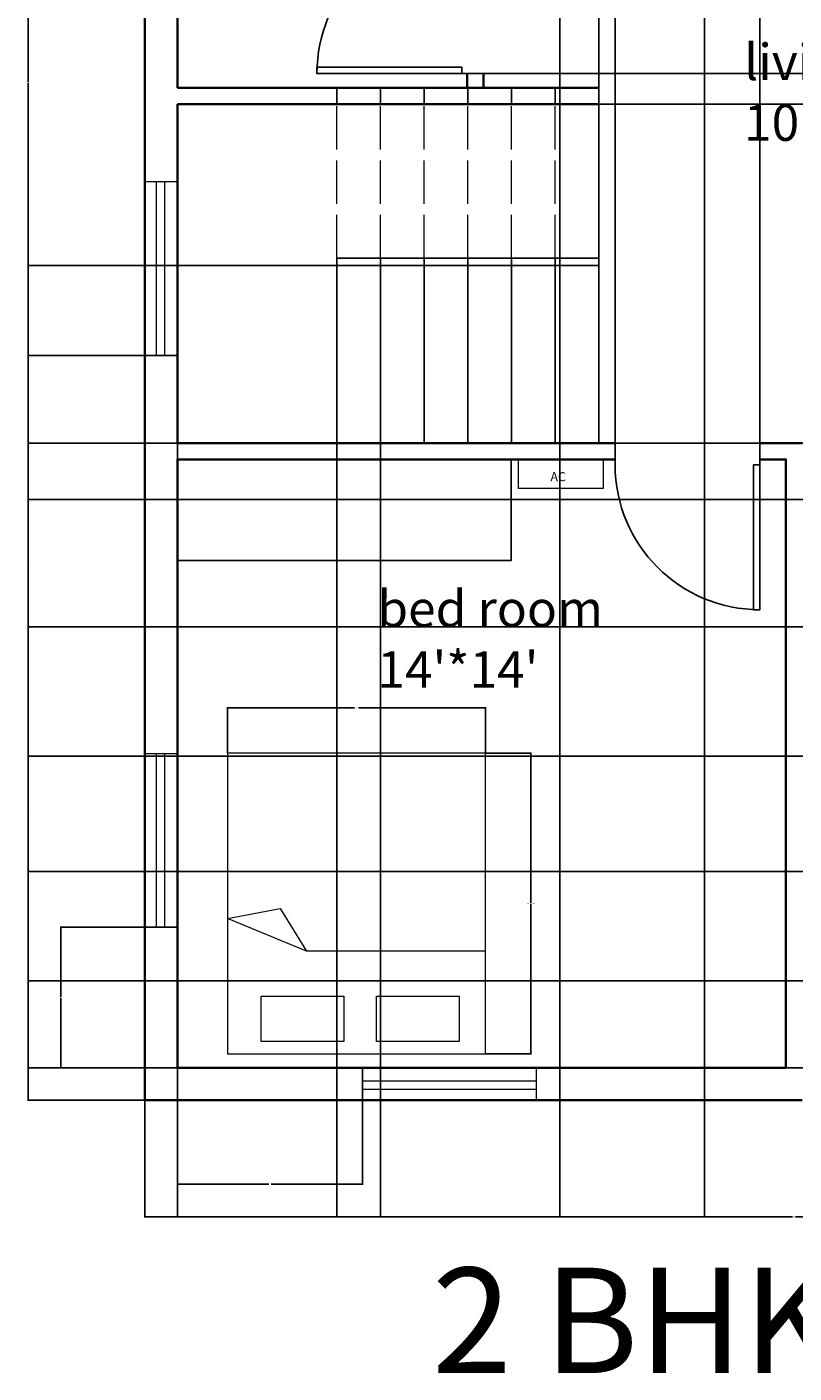
# Model space of a CAD drawing. Units: inches. Extents: x 2187 to 2611, y 763 to 1433.
# Tile 1 of 3: x 2187 to 2399, y 763 to 1135. Entities that reach past the tile are written whole.
import ezdxf

# ---------------------------------------------------------------- set-up
doc = ezdxf.new("R2010")
doc.units = ezdxf.units.IN
doc.linetypes.add('ACAD_ISO02W100', pattern=[15, 12, -3])
for name, color, linetype, lineweight in [('A-ANNO-DIMS', 2, 'Continuous', 18), ('A-ANNO-TEXT', 7, 'Continuous', 18), ('A-ANNO-TITL', 7, 'Continuous', 35), ('A-AREA-IDEN', 7, 'Continuous', 18), ('A-FLOR-CASE', 82, 'Continuous', 25), ('A-FLOR-STRS', 7, 'Continuous', 25), ('A-FLOR-STRS-OVHD', 7, 'ACAD_ISO02W100', 18), ('A-WALL', 7, 'Continuous', 35), ('DOOR', 130, 'Continuous', 25), ('FURNITURE', 82, 'Continuous', 18), ('M-HVAC-EQPM', 82, 'Continuous', 18), ('WINDOW', 50, 'Continuous', 20)]:
    doc.layers.add(name, color=color, linetype=linetype, lineweight=lineweight)
doc.styles.get("Standard").update_dxf_attribs({"font": 'arial.ttf'})
doc.dimstyles.get("Standard").update_dxf_attribs({"dimtxt": 0.18, "dimasz": 0.18, "dimexe": 0.18, "dimexo": 0.0625, "dimgap": 0.09, "dimtad": 0, "dimtih": 1, "dimtoh": 1, "dimdec": 4, "dimzin": 0, "dimdsep": 46, "dimtxsty": 'Standard', "dimcen": 0.09, "dimadec": 0, "dimazin": 0, "dimtfac": 1, "dimtdec": 4, "dimtofl": 0, "dimtmove": 0, "dimatfit": 3, "dimfxl": 1, "dimtolj": 1, "dimtzin": 0, "dimarcsym": 0})

# ---------------------------------------------------------------- blocks, each defined once
blk = doc.blocks.new('*U2')
for p, q in [((0, 0), (0, -6)), ((40, 0), (40, -6))]:
    blk.add_line(p, q)
blk.add_lwpolyline([(0, 0), (0, 40), (1.75, 40), (1.75, 0)], close=True)
blk.add_arc((0, 0), 40, 0, 90)
blk = doc.blocks.new('BED-DOUBLE')
for p, q in [((54.72, 71.29), (54.72, 21.8)), ((42.94, 14.53), (54.72, 21.8)), ((54.72, 21.8), (45.71, 0)), ((45.71, 0), (42.94, 14.53))]:
    blk.add_line(p, q)
for points in [[(83.12, 71.29), (0, 71.29), (0, 0), (83.12, 0)], [(67.19, 64.02), (79.65, 64.02), (79.65, 41.18), (67.19, 41.18)], [(67.19, 32.18), (79.65, 32.18), (79.65, 9.34), (67.19, 9.34)]]:
    blk.add_lwpolyline(points, close=True)
blk = doc.blocks.new('WIN-48IN')
for p, q in [((0, 0), (0, 9)), ((48, 0), (48, 9)), ((0, 5.37), (48, 5.37)), ((0, 3.09), (48, 3.09))]:
    blk.add_line(p, q)
blk = doc.blocks.new('*D10')
at = {"layer": 'A-ANNO-DIMS', "color": 0, "lineweight": -2, "transparency": 16777216}
for p, q in [((2313.9, 934.72), (2326.49, 934.72)), ((2326.31, 934.54), (2326.31, 893.34)), ((2326.31, 851.78), (2326.31, 892.98)), ((2313.9, 851.6), (2326.49, 851.6))]:
    blk.add_line(p, q, dxfattribs=at)
at = {"layer": 'A-ANNO-DIMS', "color": 0, "lineweight": 100, "transparency": 16777216}
for points in [[(2326.28, 934.54), (2326.34, 934.54), (2326.31, 934.72)], [(2326.28, 851.78), (2326.34, 851.78), (2326.31, 851.6)]]:
    blk.add_solid(points, dxfattribs=at)
at = {"layer": 'Defpoints', "color": 0, "lineweight": 100, "transparency": 16777216}
for p in [(2313.84, 934.72), (2313.84, 851.6), (2326.31, 851.6)]:
    blk.add_point(p, dxfattribs=at)
at = {"layer": 'A-ANNO-DIMS', "color": 0, "transparency": 16777216, "insert": (2326.31, 893.16), "char_height": 0.18, "attachment_point": 5}
blk.add_mtext('\\A1;DOUBLE BED 83 TYP.', dxfattribs=at)
blk = doc.blocks.new('*D11')
at = {"layer": 'A-ANNO-DIMS', "color": 0, "lineweight": -2, "transparency": 16777216}
for p, q in [((2242.55, 934.78), (2242.55, 947.37)), ((2242.73, 947.19), (2277.67, 947.19)), ((2313.66, 947.19), (2278.72, 947.19)), ((2313.84, 934.78), (2313.84, 947.37))]:
    blk.add_line(p, q, dxfattribs=at)
at = {"layer": 'A-ANNO-DIMS', "color": 0, "lineweight": 100, "transparency": 16777216}
for points in [[(2242.73, 947.22), (2242.73, 947.16), (2242.55, 947.19)], [(2313.66, 947.22), (2313.66, 947.16), (2313.84, 947.19)]]:
    blk.add_solid(points, dxfattribs=at)
at = {"layer": 'Defpoints', "color": 0, "lineweight": 100, "transparency": 16777216}
for p in [(2313.84, 947.19), (2242.55, 934.72), (2313.84, 934.72)]:
    blk.add_point(p, dxfattribs=at)
at = {"layer": 'A-ANNO-DIMS', "color": 0, "transparency": 16777216, "insert": (2278.2, 947.19), "char_height": 0.18, "attachment_point": 5}
blk.add_mtext('\\A1;71 TYP.', dxfattribs=at)
blk = doc.blocks.new('*D14')
at = {"layer": 'A-ANNO-DIMS', "color": 0, "lineweight": -2, "transparency": 16777216}
for p, q in [((2219.77, 838.73), (2219.77, 806.41)), ((2578.27, 838.73), (2578.27, 806.41)), ((2219.95, 806.59), (2398.62, 806.59)), ((2578.09, 806.59), (2399.41, 806.59))]:
    blk.add_line(p, q, dxfattribs=at)
at = {"layer": 'A-ANNO-DIMS', "color": 0, "lineweight": 100, "transparency": 16777216}
for points in [[(2219.95, 806.62), (2219.95, 806.56), (2219.77, 806.59)], [(2578.09, 806.62), (2578.09, 806.56), (2578.27, 806.59)]]:
    blk.add_solid(points, dxfattribs=at)
at = {"layer": 'Defpoints', "color": 0, "lineweight": 100, "transparency": 16777216}
for p in [(2219.77, 838.79), (2578.27, 838.79), (2578.27, 806.59)]:
    blk.add_point(p, dxfattribs=at)
at = {"layer": 'A-ANNO-DIMS', "color": 0, "transparency": 16777216, "insert": (2399.02, 806.59), "char_height": 0.18, "attachment_point": 5}
blk.add_mtext('\\A1;358.5', dxfattribs=at)
blk = doc.blocks.new('*D15')
at = {"layer": 'A-ANNO-DIMS', "color": 0, "lineweight": -2, "transparency": 16777216}
for p, q in [((2219.71, 1400.96), (2187.39, 1400.96)), ((2187.57, 1400.78), (2187.57, 1120.06)), ((2187.57, 838.97), (2187.57, 1119.7)), ((2219.71, 838.79), (2187.39, 838.79))]:
    blk.add_line(p, q, dxfattribs=at)
at = {"layer": 'A-ANNO-DIMS', "color": 0, "lineweight": 100, "transparency": 16777216}
for points in [[(2187.54, 1400.78), (2187.6, 1400.78), (2187.57, 1400.96)], [(2187.54, 838.97), (2187.6, 838.97), (2187.57, 838.79)]]:
    blk.add_solid(points, dxfattribs=at)
at = {"layer": 'Defpoints', "color": 0, "lineweight": 100, "transparency": 16777216}
for p in [(2187.57, 1400.96), (2219.77, 1400.96), (2219.77, 838.79)]:
    blk.add_point(p, dxfattribs=at)
at = {"layer": 'A-ANNO-DIMS', "color": 0, "transparency": 16777216, "insert": (2187.57, 1119.88), "char_height": 0.18, "attachment_point": 5}
blk.add_mtext('\\A1;562.2', dxfattribs=at)
blk = doc.blocks.new('*D20')
at = {"layer": 'A-ANNO-DIMS', "color": 0, "lineweight": -2, "transparency": 16777216}
for p, q in [((2228.71, 886.61), (2196.39, 886.61)), ((2196.57, 886.43), (2196.57, 867.38)), ((2196.57, 847.97), (2196.57, 867.02)), ((2228.71, 847.79), (2196.39, 847.79))]:
    blk.add_line(p, q, dxfattribs=at)
at = {"layer": 'A-ANNO-DIMS', "color": 0, "lineweight": 100, "transparency": 16777216}
for points in [[(2196.54, 886.43), (2196.6, 886.43), (2196.57, 886.61)], [(2196.54, 847.97), (2196.6, 847.97), (2196.57, 847.79)]]:
    blk.add_solid(points, dxfattribs=at)
at = {"layer": 'Defpoints', "color": 0, "lineweight": 100, "transparency": 16777216}
for p in [(2196.57, 886.61), (2228.77, 886.61), (2228.77, 847.79)]:
    blk.add_point(p, dxfattribs=at)
at = {"layer": 'A-ANNO-DIMS', "color": 0, "transparency": 16777216, "insert": (2196.57, 867.2), "char_height": 0.18, "attachment_point": 5}
blk.add_mtext('\\A1;38.81', dxfattribs=at)
blk = doc.blocks.new('*D21')
at = {"layer": 'A-ANNO-DIMS', "color": 0, "lineweight": -2, "transparency": 16777216}
for p, q in [((2228.77, 847.73), (2228.77, 815.41)), ((2279.87, 847.73), (2279.87, 815.41)), ((2228.95, 815.59), (2254.01, 815.59)), ((2279.69, 815.59), (2254.63, 815.59))]:
    blk.add_line(p, q, dxfattribs=at)
at = {"layer": 'A-ANNO-DIMS', "color": 0, "lineweight": 100, "transparency": 16777216}
for points in [[(2228.95, 815.62), (2228.95, 815.56), (2228.77, 815.59)], [(2279.69, 815.62), (2279.69, 815.56), (2279.87, 815.59)]]:
    blk.add_solid(points, dxfattribs=at)
at = {"layer": 'Defpoints', "color": 0, "lineweight": 100, "transparency": 16777216}
for p in [(2228.77, 847.79), (2279.87, 847.79), (2228.77, 815.59)]:
    blk.add_point(p, dxfattribs=at)
at = {"layer": 'A-ANNO-DIMS', "color": 0, "transparency": 16777216, "insert": (2254.32, 815.59), "char_height": 0.18, "attachment_point": 5}
blk.add_mtext('\\A1;51.1', dxfattribs=at)
blk = doc.blocks.new('*D28')
at = {"layer": 'A-ANNO-DIMS', "color": 0, "lineweight": -2, "transparency": 16777216}
for p, q in [((2349.61, 1016.11), (2349.61, 1433.34)), ((2349.79, 1433.16), (2369.39, 1433.16)), ((2389.43, 1433.16), (2369.83, 1433.16)), ((2389.61, 1016.11), (2389.61, 1433.34))]:
    blk.add_line(p, q, dxfattribs=at)
at = {"layer": 'A-ANNO-DIMS', "color": 0, "lineweight": 100, "transparency": 16777216}
for points in [[(2349.79, 1433.19), (2349.79, 1433.13), (2349.61, 1433.16)], [(2389.43, 1433.19), (2389.43, 1433.13), (2389.61, 1433.16)]]:
    blk.add_solid(points, dxfattribs=at)
at = {"layer": 'Defpoints', "color": 0, "lineweight": 100, "transparency": 16777216}
for p in [(2389.61, 1433.16), (2349.61, 1016.04), (2389.61, 1016.04)]:
    blk.add_point(p, dxfattribs=at)
at = {"layer": 'A-ANNO-DIMS', "color": 0, "transparency": 16777216, "insert": (2369.61, 1433.16), "char_height": 0.18, "attachment_point": 5}
blk.add_mtext('\\A1;40', dxfattribs=at)
blk = doc.blocks.new('*D29')
at = {"layer": 'A-ANNO-DIMS', "color": 0, "lineweight": -2, "transparency": 16777216}
for p, q in [((2447.71, 1004.76), (2187.39, 1004.76)), ((2187.57, 1004.58), (2187.57, 987.33)), ((2187.57, 969.72), (2187.57, 986.97)), ((2447.71, 969.54), (2187.39, 969.54))]:
    blk.add_line(p, q, dxfattribs=at)
at = {"layer": 'A-ANNO-DIMS', "color": 0, "lineweight": 100, "transparency": 16777216}
for points in [[(2187.54, 1004.58), (2187.6, 1004.58), (2187.57, 1004.76)], [(2187.54, 969.72), (2187.6, 969.72), (2187.57, 969.54)]]:
    blk.add_solid(points, dxfattribs=at)
at = {"layer": 'Defpoints', "color": 0, "lineweight": 100, "transparency": 16777216}
for p in [(2187.57, 1004.76), (2447.77, 1004.76), (2447.77, 969.54)]:
    blk.add_point(p, dxfattribs=at)
at = {"layer": 'A-ANNO-DIMS', "color": 0, "transparency": 16777216, "insert": (2187.57, 987.15), "char_height": 0.18, "attachment_point": 5}
blk.add_mtext('\\A1;35.22', dxfattribs=at)
blk = doc.blocks.new('*D30')
at = {"layer": 'A-ANNO-DIMS', "color": 0, "lineweight": -2, "transparency": 16777216}
for p, q in [((2334.33, 1219.4), (2334.33, 806.41)), ((2374.33, 1219.4), (2374.33, 806.41)), ((2334.51, 806.59), (2354.11, 806.59)), ((2374.15, 806.59), (2354.56, 806.59))]:
    blk.add_line(p, q, dxfattribs=at)
at = {"layer": 'A-ANNO-DIMS', "color": 0, "lineweight": 100, "transparency": 16777216}
for points in [[(2334.51, 806.62), (2334.51, 806.56), (2334.33, 806.59)], [(2374.15, 806.62), (2374.15, 806.56), (2374.33, 806.59)]]:
    blk.add_solid(points, dxfattribs=at)
at = {"layer": 'Defpoints', "color": 0, "lineweight": 100, "transparency": 16777216}
for p in [(2334.33, 1219.46), (2374.33, 1219.46), (2374.33, 806.59)]:
    blk.add_point(p, dxfattribs=at)
at = {"layer": 'A-ANNO-DIMS', "color": 0, "transparency": 16777216, "insert": (2354.33, 806.59), "char_height": 0.18, "attachment_point": 5}
blk.add_mtext('\\A1;40', dxfattribs=at)
blk = doc.blocks.new('*D31')
at = {"layer": 'A-ANNO-DIMS', "color": 0, "lineweight": -2, "transparency": 16777216}
for p, q in [((2313.33, 1162.4), (2610.65, 1162.4)), ((2610.47, 1162.22), (2610.47, 1142.58)), ((2610.47, 1122.58), (2610.47, 1142.22)), ((2313.33, 1122.4), (2610.65, 1122.4))]:
    blk.add_line(p, q, dxfattribs=at)
at = {"layer": 'A-ANNO-DIMS', "color": 0, "lineweight": 100, "transparency": 16777216}
for points in [[(2610.44, 1162.22), (2610.5, 1162.22), (2610.47, 1162.4)], [(2610.44, 1122.58), (2610.5, 1122.58), (2610.47, 1122.4)]]:
    blk.add_solid(points, dxfattribs=at)
at = {"layer": 'Defpoints', "color": 0, "lineweight": 100, "transparency": 16777216}
for p in [(2313.27, 1162.4), (2610.47, 1162.4), (2313.27, 1122.4)]:
    blk.add_point(p, dxfattribs=at)
at = {"layer": 'A-ANNO-DIMS', "color": 0, "transparency": 16777216, "insert": (2610.47, 1142.4), "char_height": 0.18, "attachment_point": 5}
blk.add_mtext('\\A1;40', dxfattribs=at)
blk = doc.blocks.new('*D34')
at = {"layer": 'A-ANNO-DIMS', "color": 0, "lineweight": -2, "transparency": 16777216}
for p, q in [((2449.71, 871.79), (2187.39, 871.79)), ((2187.57, 871.61), (2187.57, 859.97)), ((2187.57, 847.97), (2187.57, 859.61)), ((2449.71, 847.79), (2187.39, 847.79))]:
    blk.add_line(p, q, dxfattribs=at)
at = {"layer": 'A-ANNO-DIMS', "color": 0, "lineweight": 100, "transparency": 16777216}
for points in [[(2187.54, 871.61), (2187.6, 871.61), (2187.57, 871.79)], [(2187.54, 847.97), (2187.6, 847.97), (2187.57, 847.79)]]:
    blk.add_solid(points, dxfattribs=at)
at = {"layer": 'Defpoints', "color": 0, "lineweight": 100, "transparency": 16777216}
for p in [(2187.57, 871.79), (2449.78, 871.79), (2449.78, 847.79)]:
    blk.add_point(p, dxfattribs=at)
at = {"layer": 'A-ANNO-DIMS', "color": 0, "transparency": 16777216, "insert": (2187.57, 859.79), "char_height": 0.18, "attachment_point": 5}
blk.add_mtext('\\A1;24', dxfattribs=at)
blk = doc.blocks.new('*D43')
at = {"layer": 'A-ANNO-DIMS', "color": 0, "lineweight": -2, "transparency": 16777216}
for p, q in [((2546.13, 933.87), (2187.39, 933.87)), ((2187.57, 933.69), (2187.57, 918.13)), ((2187.57, 902.21), (2187.57, 917.77)), ((2546.13, 902.03), (2187.39, 902.03))]:
    blk.add_line(p, q, dxfattribs=at)
at = {"layer": 'A-ANNO-DIMS', "color": 0, "lineweight": 100, "transparency": 16777216}
for points in [[(2187.54, 933.69), (2187.6, 933.69), (2187.57, 933.87)], [(2187.54, 902.21), (2187.6, 902.21), (2187.57, 902.03)]]:
    blk.add_solid(points, dxfattribs=at)
at = {"layer": 'Defpoints', "color": 0, "lineweight": 100, "transparency": 16777216}
for p in [(2187.57, 933.87), (2546.19, 933.87), (2546.19, 902.03)]:
    blk.add_point(p, dxfattribs=at)
at = {"layer": 'A-ANNO-DIMS', "color": 0, "transparency": 16777216, "insert": (2187.57, 917.95), "char_height": 0.18, "attachment_point": 5}
blk.add_mtext('\\A1;31.837', dxfattribs=at)
blk = doc.blocks.new('*D44')
at = {"layer": 'A-ANNO-DIMS', "color": 0, "lineweight": -2, "transparency": 16777216}
for p, q in [((2228.77, 1118.52), (2228.77, 1433.34)), ((2228.95, 1433.16), (2286.53, 1433.16)), ((2344.89, 1433.16), (2287.3, 1433.16)), ((2345.07, 1118.52), (2345.07, 1433.34))]:
    blk.add_line(p, q, dxfattribs=at)
at = {"layer": 'A-ANNO-DIMS', "color": 0, "lineweight": 100, "transparency": 16777216}
for points in [[(2228.95, 1433.19), (2228.95, 1433.13), (2228.77, 1433.16)], [(2344.89, 1433.19), (2344.89, 1433.13), (2345.07, 1433.16)]]:
    blk.add_solid(points, dxfattribs=at)
at = {"layer": 'Defpoints', "color": 0, "lineweight": 100, "transparency": 16777216}
for p in [(2345.07, 1433.16), (2228.77, 1118.46), (2345.07, 1118.46)]:
    blk.add_point(p, dxfattribs=at)
at = {"layer": 'A-ANNO-DIMS', "color": 0, "transparency": 16777216, "insert": (2286.92, 1433.16), "char_height": 0.18, "attachment_point": 5}
blk.add_mtext('\\A1;116.3', dxfattribs=at)
blk = doc.blocks.new('*D45')
at = {"layer": 'A-ANNO-DIMS', "color": 0, "lineweight": -2, "transparency": 16777216}
for p, q in [((2345.13, 1113.96), (2610.65, 1113.96)), ((2610.47, 1113.78), (2610.47, 1067.31)), ((2610.47, 1020.47), (2610.47, 1066.94)), ((2345.13, 1020.29), (2610.65, 1020.29))]:
    blk.add_line(p, q, dxfattribs=at)
at = {"layer": 'A-ANNO-DIMS', "color": 0, "lineweight": 100, "transparency": 16777216}
for points in [[(2610.44, 1113.78), (2610.5, 1113.78), (2610.47, 1113.96)], [(2610.44, 1020.47), (2610.5, 1020.47), (2610.47, 1020.29)]]:
    blk.add_solid(points, dxfattribs=at)
at = {"layer": 'Defpoints', "color": 0, "lineweight": 100, "transparency": 16777216}
for p in [(2345.07, 1113.96), (2610.47, 1113.96), (2345.07, 1020.29)]:
    blk.add_point(p, dxfattribs=at)
at = {"layer": 'A-ANNO-DIMS', "color": 0, "transparency": 16777216, "insert": (2610.47, 1067.13), "char_height": 0.18, "attachment_point": 5}
blk.add_mtext('\\A1;93.67', dxfattribs=at)
blk = doc.blocks.new('*D46')
at = {"layer": 'A-ANNO-DIMS', "color": 0, "lineweight": -2, "transparency": 16777216}
for p, q in [((2228.77, 1020.23), (2228.77, 806.41)), ((2272.77, 1020.23), (2272.77, 806.41)), ((2228.95, 806.59), (2250.55, 806.59)), ((2272.59, 806.59), (2250.99, 806.59))]:
    blk.add_line(p, q, dxfattribs=at)
at = {"layer": 'A-ANNO-DIMS', "color": 0, "lineweight": 100, "transparency": 16777216}
for points in [[(2228.95, 806.62), (2228.95, 806.56), (2228.77, 806.59)], [(2272.59, 806.62), (2272.59, 806.56), (2272.77, 806.59)]]:
    blk.add_solid(points, dxfattribs=at)
at = {"layer": 'Defpoints', "color": 0, "lineweight": 100, "transparency": 16777216}
for p in [(2228.77, 1020.29), (2272.77, 1020.29), (2272.77, 806.59)]:
    blk.add_point(p, dxfattribs=at)
at = {"layer": 'A-ANNO-DIMS', "color": 0, "transparency": 16777216, "insert": (2250.77, 806.59), "char_height": 0.18, "attachment_point": 5}
blk.add_mtext('\\A1;44', dxfattribs=at)
blk = doc.blocks.new('*D47')
at = {"layer": 'A-ANNO-DIMS', "color": 0, "lineweight": -2, "transparency": 16777216}
for p, q in [((2272.77, 1020.23), (2272.77, 806.41)), ((2284.82, 1020.23), (2284.82, 806.41)), ((2272.95, 806.59), (2278.41, 806.59)), ((2284.64, 806.59), (2279.18, 806.59))]:
    blk.add_line(p, q, dxfattribs=at)
at = {"layer": 'A-ANNO-DIMS', "color": 0, "lineweight": 100, "transparency": 16777216}
for points in [[(2272.95, 806.62), (2272.95, 806.56), (2272.77, 806.59)], [(2284.64, 806.62), (2284.64, 806.56), (2284.82, 806.59)]]:
    blk.add_solid(points, dxfattribs=at)
at = {"layer": 'Defpoints', "color": 0, "lineweight": 100, "transparency": 16777216}
for p in [(2272.77, 1020.29), (2284.82, 1020.29), (2284.82, 806.59)]:
    blk.add_point(p, dxfattribs=at)
at = {"layer": 'A-ANNO-DIMS', "color": 0, "transparency": 16777216, "insert": (2278.79, 806.59), "char_height": 0.18, "attachment_point": 5}
blk.add_mtext('\\A1;12.05', dxfattribs=at)
blk = doc.blocks.new('*D48')
at = {"layer": 'A-ANNO-DIMS', "color": 0, "lineweight": -2, "transparency": 16777216}
for p, q in [((2272.71, 1069.38), (2187.39, 1069.38)), ((2187.57, 1069.2), (2187.57, 1045.02)), ((2187.57, 1020.47), (2187.57, 1044.65)), ((2272.71, 1020.29), (2187.39, 1020.29))]:
    blk.add_line(p, q, dxfattribs=at)
at = {"layer": 'A-ANNO-DIMS', "color": 0, "lineweight": 100, "transparency": 16777216}
for points in [[(2187.54, 1069.2), (2187.6, 1069.2), (2187.57, 1069.38)], [(2187.54, 1020.47), (2187.6, 1020.47), (2187.57, 1020.29)]]:
    blk.add_solid(points, dxfattribs=at)
at = {"layer": 'Defpoints', "color": 0, "lineweight": 100, "transparency": 16777216}
for p in [(2187.57, 1069.38), (2272.77, 1069.38), (2272.77, 1020.29)]:
    blk.add_point(p, dxfattribs=at)
at = {"layer": 'A-ANNO-DIMS', "color": 0, "transparency": 16777216, "insert": (2187.57, 1044.84), "char_height": 0.18, "attachment_point": 5}
blk.add_mtext('\\A1;49.08', dxfattribs=at)
blk = doc.blocks.new('*D49')
at = {"layer": 'A-ANNO-DIMS', "color": 0, "lineweight": -2, "transparency": 16777216}
for p, q in [((2228.71, 1044.55), (2187.39, 1044.55)), ((2187.57, 1044.37), (2187.57, 1032.6)), ((2187.57, 1020.47), (2187.57, 1032.24)), ((2228.71, 1020.29), (2187.39, 1020.29))]:
    blk.add_line(p, q, dxfattribs=at)
at = {"layer": 'A-ANNO-DIMS', "color": 0, "lineweight": 100, "transparency": 16777216}
for points in [[(2187.54, 1044.37), (2187.6, 1044.37), (2187.57, 1044.55)], [(2187.54, 1020.47), (2187.6, 1020.47), (2187.57, 1020.29)]]:
    blk.add_solid(points, dxfattribs=at)
at = {"layer": 'Defpoints', "color": 0, "lineweight": 100, "transparency": 16777216}
for p in [(2187.57, 1044.55), (2228.77, 1044.55), (2228.77, 1020.29)]:
    blk.add_point(p, dxfattribs=at)
at = {"layer": 'A-ANNO-DIMS', "color": 0, "transparency": 16777216, "insert": (2187.57, 1032.42), "char_height": 0.18, "attachment_point": 5}
blk.add_mtext('\\A1;24.25', dxfattribs=at)

msp = doc.modelspace()

# ---------------------------------------------------------------- linework, layer by layer
at = {"layer": 'A-FLOR-CASE'}
msp.add_lwpolyline([(2228.7681, 1015.7937), (2320.9466, 1015.7937), (2320.9466, 987.9063), (2228.7681, 987.9063)], close=True, dxfattribs=at)
at = {"layer": 'A-FLOR-STRS'}
for p, q in [((2272.7686, 1118.4602), (2272.7686, 1113.9602)), ((2284.8182, 1118.4602), (2284.8182, 1113.9602)), ((2296.8678, 1118.4602), (2296.8678, 1113.9602)), ((2308.9175, 1118.4602), (2308.9175, 1113.9602)), ((2320.9671, 1118.4602), (2320.9671, 1113.9602)), ((2333.0167, 1118.4602), (2333.0167, 1113.9602)), ((2345.0663, 1113.9602), (2345.0663, 1118.4602)), ((2345.0663, 1069.377), (2345.0663, 1118.4602)), ((2345.0663, 1118.4602), (2345.0663, 1020.2937)), ((2228.7681, 1113.9602), (2228.7681, 1020.2937)), ((2272.7686, 1071.377), (2345.0663, 1071.377)), ((2272.7686, 1071.377), (2272.7686, 1020.2937)), ((2284.8182, 1071.377), (2284.8182, 1020.2937)), ((2296.8678, 1071.377), (2296.8678, 1020.2937)), ((2308.9175, 1071.377), (2308.9175, 1020.2937)), ((2320.9671, 1071.377), (2320.9671, 1020.2937)), ((2333.0167, 1071.377), (2333.0167, 1020.2937)), ((2272.7686, 1069.377), (2345.0663, 1069.377))]:
    msp.add_line(p, q, dxfattribs=at)
at = {"layer": 'A-FLOR-STRS-OVHD'}
for p, q in [((2272.7686, 1071.377), (2272.7686, 1113.9602)), ((2284.8182, 1071.377), (2284.8182, 1113.9602)), ((2296.8678, 1071.377), (2296.8678, 1113.9602)), ((2308.9175, 1071.377), (2308.9175, 1113.9602)), ((2320.9671, 1071.377), (2320.9671, 1113.9602)), ((2333.0167, 1071.377), (2333.0167, 1113.9602))]:
    msp.add_line(p, q, dxfattribs=at)
at = {"layer": 'A-WALL'}
for p, q in [((2219.7681, 1118.4602), (2219.7681, 1223.9602)), ((2228.7681, 1118.4602), (2228.7681, 1219.4602)), ((2308.7681, 1122.3972), (2308.7681, 1118.4602)), ((2313.2681, 1122.3972), (2313.2681, 1118.4602)), ((2219.7681, 1020.2937), (2219.7681, 1118.4602)), ((2228.7681, 1118.4602), (2345.0663, 1118.4602)), ((2228.7681, 1020.2937), (2228.7681, 1113.9602)), ((2228.7681, 1113.9602), (2345.0663, 1113.9602)), ((2219.7681, 1020.2937), (2219.7681, 838.7937)), ((2228.7681, 1020.2937), (2349.6096, 1020.2937)), ((2389.6096, 1020.2937), (2401.2681, 1020.2937)), ((2228.7681, 1015.7937), (2349.6096, 1015.7937)), ((2228.7681, 1015.7937), (2228.7681, 847.7937)), ((2389.6096, 1015.7937), (2396.7681, 1015.7937)), ((2396.7681, 847.7937), (2396.7681, 1015.7937)), ((2228.7681, 847.7937), (2396.7681, 847.7937)), ((2219.7681, 838.7937), (2401.2681, 838.7937))]:
    msp.add_line(p, q, dxfattribs=at)
msp.add_lwpolyline([(2349.6096, 1015.7937), (2228.7681, 1015.7937), (2228.7681, 847.7937), (2396.7681, 847.7937), (2396.7681, 1015.7937), (2389.6096, 1015.7937)], dxfattribs=at)
at = {"layer": 'M-HVAC-EQPM'}
msp.add_lwpolyline([(2322.9531, 1015.7937), (2346.3099, 1015.7937), (2346.3099, 1007.7676), (2322.9531, 1007.7676)], close=True, dxfattribs=at)

# ---------------------------------------------------------------- block references
at = {"layer": 'DOOR'}
for p, rotation in [((2307.2681, 1122.3972), 90.00000000000003), ((2389.6096, 1014.2937), 180)]:
    msp.add_blockref('*U2', p, dxfattribs=dict(at, rotation=rotation))
at = {"layer": 'FURNITURE', "rotation": 270.0000000000003}
msp.add_blockref('BED-DOUBLE', (2242.5534, 934.7199), dxfattribs=at)
at = {"layer": 'WINDOW', "rotation": 270.0000000000009}
for p in [(2219.7681, 1092.5453), (2219.7681, 934.6052)]:
    msp.add_blockref('WIN-48IN', p, dxfattribs=at)
at = {"layer": 'WINDOW'}
msp.add_blockref('WIN-48IN', (2279.8729, 838.7937), dxfattribs=at)

# ---------------------------------------------------------------- texts
at = {"layer": 'A-ANNO-TEXT', "insert": (2331.7535, 1012.2931), "char_height": 2.5, "attachment_point": 1}
msp.add_mtext_dynamic_manual_height_columns('AC', width=7.404151, gutter_width=12.5, heights=[0], dxfattribs=at)
at = {"layer": 'A-ANNO-TITL', "insert": (2299.0368, 792.5375), "char_height": 29.09468, "attachment_point": 1}
msp.add_mtext_dynamic_manual_height_columns('2 BHK PLAN', width=464.084837, gutter_width=145.4734, heights=[0], dxfattribs=at)
at = {"layer": 'A-AREA-IDEN', "attachment_point": 1}
for s, insert, char_height in [('living/dining\\P10\'4"*29\'3"', (2385.2182, 1130.6372), 10.056757), ("bed room\\P14'*14'", (2283.9581, 979.5996), 10.05676)]:
    msp.add_mtext_dynamic_manual_height_columns(s, width=160.413815, gutter_width=50.2838, heights=[0], dxfattribs=dict(at, insert=insert, char_height=char_height))

# ---------------------------------------------------------------- dimensions: what is measured, and where the dimension line sits
at = {"layer": 'A-ANNO-DIMS'}
for base, p1, p2, override, picture, middle in [((2345.0663, 1433.1602), (2228.7681, 1118.4602), (2345.0663, 1118.4602), {"dimdec": 1, "dimlfac": 1, "dimrnd": 0, "dimzin": 0, "dimdsep": 46, "dimlunit": 2}, '*D44', (2286.9172, 1433.1602)), ((2389.6096, 1433.1602), (2349.6096, 1016.0437), (2389.6096, 1016.0437), {"dimdec": 0, "dimlfac": 1, "dimrnd": 0, "dimzin": 0, "dimdsep": 46, "dimlunit": 2}, '*D28', (2369.6096, 1433.1602)), ((2374.3333, 806.5937), (2334.3333, 1219.4602), (2374.3333, 1219.4602), {"dimdec": 0, "dimlfac": 1, "dimrnd": 0, "dimzin": 0, "dimdsep": 46, "dimlunit": 2}, '*D30', (2354.3333, 806.5937)), ((2272.7686, 806.5937), (2228.7681, 1020.2937), (2272.7686, 1020.2937), {"dimdec": 0, "dimlfac": 1, "dimrnd": 0, "dimzin": 0, "dimdsep": 46, "dimlunit": 2}, '*D46', (2250.7683, 806.5937)), ((2284.8182, 806.5937), (2272.7686, 1020.2937), (2284.8182, 1020.2937), {"dimdec": 2, "dimlfac": 1, "dimrnd": 0, "dimzin": 0, "dimdsep": 46, "dimlunit": 2}, '*D47', (2278.7934, 806.5937)), ((2578.2681, 806.5937), (2219.7681, 838.7937), (2578.2681, 838.7937), {"dimdec": 1, "dimlfac": 1, "dimrnd": 0, "dimzin": 0, "dimdsep": 46, "dimlunit": 2}, '*D14', (2399.0181, 806.5937))]:
    dim = msp.add_linear_dim(base=base, p1=p1, p2=p2, dimstyle='Standard', override=override, dxfattribs=at)
    dim.commit()
    dim.dimension.update_dxf_attribs({"geometry": picture, "text_midpoint": middle})
for base, p1, p2, angle, override, picture, middle in [((2187.5681, 1400.9602), (2219.7681, 838.7937), (2219.7681, 1400.9602), 90, {"dimdec": 1, "dimlfac": 1, "dimrnd": 0, "dimzin": 0, "dimdsep": 46, "dimlunit": 2}, '*D15', (2187.5681, 1119.877)), ((2610.4681, 1162.3972), (2313.2681, 1122.3972), (2313.2681, 1162.3972), 90, {"dimdec": 0, "dimlfac": 1, "dimrnd": 0, "dimzin": 0, "dimdsep": 46, "dimlunit": 2}, '*D31', (2610.4681, 1142.3972)), ((2610.4681, 1113.9602), (2345.0663, 1020.2937), (2345.0663, 1113.9602), 90, {"dimdec": 2, "dimlfac": 1, "dimrnd": 0, "dimzin": 0, "dimdsep": 46, "dimlunit": 2}, '*D45', (2610.4681, 1067.127)), ((2187.5681, 1069.377), (2272.7686, 1020.2937), (2272.7686, 1069.377), 90, {"dimdec": 2, "dimlfac": 1, "dimrnd": 0, "dimzin": 0, "dimdsep": 46, "dimlunit": 2}, '*D48', (2187.5681, 1044.8353)), ((2187.5681, 1044.5453), (2228.7681, 1020.2937), (2228.7681, 1044.5453), 90, {"dimdec": 2, "dimlfac": 1, "dimrnd": 0, "dimzin": 0, "dimdsep": 46, "dimlunit": 2}, '*D49', (2187.5681, 1032.4195)), ((2187.5681, 1004.7585), (2447.7681, 969.5415), (2447.7681, 1004.7585), 90, {"dimdec": 2, "dimlfac": 1, "dimrnd": 0, "dimzin": 0, "dimdsep": 46, "dimlunit": 2}, '*D29', (2187.5681, 987.15)), ((2187.5681, 933.8683), (2546.1934, 902.0317), (2546.1934, 933.8683), 90, {"dimdec": 3, "dimlfac": 1, "dimrnd": 0, "dimzin": 0, "dimdsep": 46, "dimlunit": 2}, '*D43', (2187.5681, 917.95)), ((2196.5681, 886.6052), (2228.7681, 847.7937), (2228.7681, 886.6052), 90, {"dimdec": 2, "dimlfac": 1, "dimrnd": 0, "dimzin": 0, "dimdsep": 46, "dimlunit": 2}, '*D20', (2196.5681, 867.1995)), ((2187.5681, 871.7937), (2449.7774, 847.7937), (2449.7774, 871.7937), 90, {"dimdec": 0, "dimlfac": 1, "dimrnd": 0, "dimzin": 0, "dimdsep": 46, "dimlunit": 2}, '*D34', (2187.5681, 859.7937)), ((2228.7681, 815.5937), (2279.8729, 847.7937), (2228.7681, 847.7937), 180, {"dimdec": 1, "dimlfac": 1, "dimrnd": 0, "dimzin": 0, "dimdsep": 46, "dimlunit": 2}, '*D21', (2254.3205, 815.5937))]:
    dim = msp.add_linear_dim(base=base, p1=p1, p2=p2, angle=angle, dimstyle='Standard', override=override, dxfattribs=at)
    dim.commit()
    dim.dimension.update_dxf_attribs({"geometry": picture, "text_midpoint": middle})
for base, p1, p2, angle, text, picture, middle in [((2313.8389, 947.1875), (2242.5534, 934.7199), (2313.8389, 934.7199), 0, '<> TYP.', '*D11', (2278.1962, 947.1875)), ((2326.3066, 851.6023), (2313.8389, 934.7199), (2313.8389, 851.6023), 270, 'DOUBLE BED <> TYP.', '*D10', (2326.3066, 893.1611))]:
    dim = msp.add_linear_dim(base=base, p1=p1, p2=p2, angle=angle, text=text, dimstyle='Standard', override={"dimdec": 0, "dimlfac": 1, "dimrnd": 0, "dimzin": 0, "dimdsep": 46, "dimlunit": 2}, dxfattribs=at)
    dim.commit()
    dim.dimension.update_dxf_attribs({"geometry": picture, "text_midpoint": middle})

doc.saveas('drawing.dxf')
